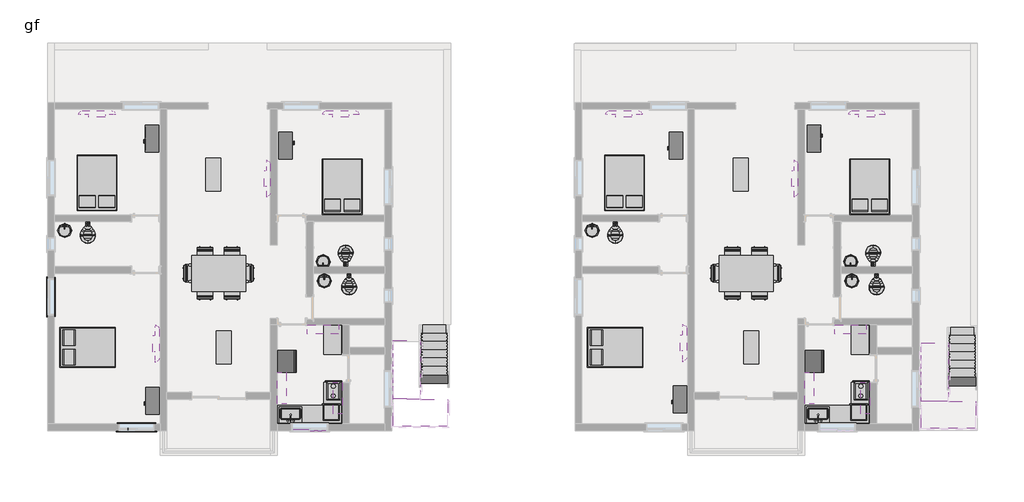
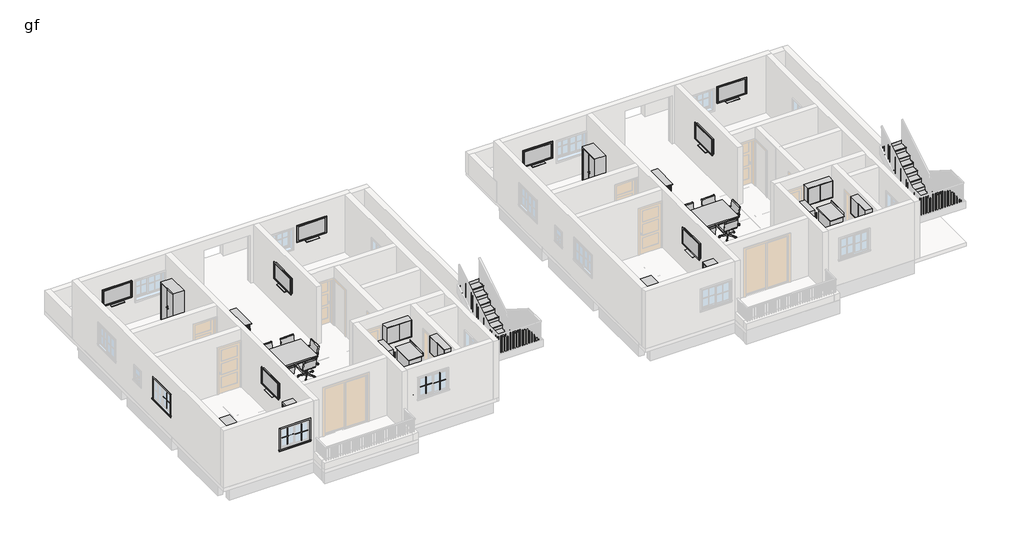
# One storey, part 7 of 8: 56 furniture elements, 23 proxies, 14 flow terminals, 4 stair flights, 2 slabs.
"""IFC4 building model written with IfcOpenShell, lengths in millimetres."""

from ifc_helpers import new_model, si_unit, origin, place, context, project, spatial, transform, mapped, element, save
from components import proxy_3c1fa1d0, proxy_caef4acf, muntin_pattern_2x2_muntin_pattern_2x2_0ac132d2, muntin_pattern_2x2_muntin_pattern_2x2_1fb5fae3, proxy_68898770, proxy_19935bb1, trim_window_exterior_flat_with_sill_c4e67c73, trim_window_exterior_flat_with_sill_729ce974, trim_window_interior_flat_picture_frame_cf1733af, trim_window_interior_flat_picture_frame_5593adf3, flow_terminal_4d548711, flow_terminal_a43f4bde, flow_terminal_3100e559, furniture_6369f5ad, furniture_f415afdb, furniture_97fe820d, furniture_b58f7881, furniture_d3d70ab1, chair_task_chair_task_b7f3823b, chair_task_arms_chair_task_arms_fa5a08ef, furniture_47cc8d9a, furniture_d87d408b, furniture_e7d75d8c, furniture_0b81fedb, furniture_74675f9f, furniture_0bcc43ae, upper_cabinet_sliding_double_door_wall_3e092c2a, non_monolithic_landing_f4ee6888, non_monolithic_landing_6912f083, stair_flight_61f47217, stair_flight_d9814c51, stair_flight_2edfd720, stair_flight_75ff7960

model = new_model("IFC4")

# Units and contexts
model_context = context("Model", 3, world=origin())
ifc_project = project(units=[si_unit("LENGTHUNIT", "METRE", prefix="MILLI")], contexts=[model_context])

# Site, building, storey
site = spatial("IfcSite", under=ifc_project)
building = spatial("IfcBuilding", under=site)
storey = spatial("IfcBuildingStorey", under=building, Name="gf", Elevation=609.6)

# Proxies
placement = place(None, origin())
proxy_shape = proxy_3c1fa1d0(model_context)
element("IfcBuildingElementProxy", 1, Name="Cook Top-2 Unit : 12\" x 18\" 2", ObjectType="Cook Top-2 Unit : 12\" x 18\" 2", at=placement, inside=storey, context=model_context, shape_type="MappedRepresentation", body=[
    mapped(proxy_shape, transform((-6699.3993763, -3292.5061971, 609.6), x_axis=(1.0, 0.0, 0.0), y_axis=(0.0, 1.0, 0.0), z_axis=(0.0, 0.0, 1.0))),
])
element("IfcBuildingElementProxy", 2, Name="Cook Top-2 Unit : 12\" x 18\" 2", ObjectType="Cook Top-2 Unit : 12\" x 18\" 2", at=placement, inside=storey, context=model_context, shape_type="MappedRepresentation", body=[
    mapped(proxy_shape, transform((11175.1761273, -3292.5061971, 609.6), x_axis=(1.0, 0.0, 0.0), y_axis=(0.0, 1.0, 0.0), z_axis=(0.0, 0.0, 1.0))),
])
proxy_2_shape = proxy_caef4acf(model_context)
element("IfcBuildingElementProxy", 3, Name="Cook Top-2 Unit : 16\" x 22\"", ObjectType="Cook Top-2 Unit : 16\" x 22\"", at=placement, inside=storey, context=model_context, shape_type="MappedRepresentation", body=[
    mapped(proxy_2_shape, transform((-6775.5993763, -4038.6311971, 609.6), x_axis=(1.0, 0.0, 0.0), y_axis=(0.0, 1.0, 0.0), z_axis=(0.0, 0.0, 1.0))),
])
element("IfcBuildingElementProxy", 4, Name="Cook Top-2 Unit : 16\" x 22\"", ObjectType="Cook Top-2 Unit : 16\" x 22\"", at=placement, inside=storey, context=model_context, shape_type="MappedRepresentation", body=[
    mapped(proxy_2_shape, transform((-6864.4993763, -4089.4311971, 609.6), x_axis=(1.0, 0.0, 0.0), y_axis=(0.0, 1.0, 0.0), z_axis=(0.0, 0.0, 1.0))),
])
element("IfcBuildingElementProxy", 5, Name="Cook Top-2 Unit : 16\" x 22\"", ObjectType="Cook Top-2 Unit : 16\" x 22\"", at=placement, inside=storey, context=model_context, shape_type="MappedRepresentation", body=[
    mapped(proxy_2_shape, transform((-6699.3993763, -3340.1311971, 609.6), x_axis=(1.0, 0.0, 0.0), y_axis=(0.0, 1.0, 0.0), z_axis=(0.0, 0.0, 1.0))),
])
element("IfcBuildingElementProxy", 6, Name="Cook Top-2 Unit : 16\" x 22\"", ObjectType="Cook Top-2 Unit : 16\" x 22\"", at=placement, inside=storey, context=model_context, shape_type="MappedRepresentation", body=[
    mapped(proxy_2_shape, transform((-6737.4993763, -3556.0311971, 609.6), x_axis=(1.0, 0.0, 0.0), y_axis=(0.0, 1.0, 0.0), z_axis=(0.0, 0.0, 1.0))),
])
element("IfcBuildingElementProxy", 7, Name="Cook Top-2 Unit : 16\" x 22\"", ObjectType="Cook Top-2 Unit : 16\" x 22\"", at=placement, inside=storey, context=model_context, shape_type="MappedRepresentation", body=[
    mapped(proxy_2_shape, transform((11098.9761273, -4038.6311971, 609.6), x_axis=(1.0, 0.0, 0.0), y_axis=(0.0, 1.0, 0.0), z_axis=(0.0, 0.0, 1.0))),
])
element("IfcBuildingElementProxy", 8, Name="Cook Top-2 Unit : 16\" x 22\"", ObjectType="Cook Top-2 Unit : 16\" x 22\"", at=placement, inside=storey, context=model_context, shape_type="MappedRepresentation", body=[
    mapped(proxy_2_shape, transform((11010.0761273, -4089.4311971, 609.6), x_axis=(1.0, 0.0, 0.0), y_axis=(0.0, 1.0, 0.0), z_axis=(0.0, 0.0, 1.0))),
])
element("IfcBuildingElementProxy", 9, Name="Cook Top-2 Unit : 16\" x 22\"", ObjectType="Cook Top-2 Unit : 16\" x 22\"", at=placement, inside=storey, context=model_context, shape_type="MappedRepresentation", body=[
    mapped(proxy_2_shape, transform((11175.1761273, -3340.1311971, 609.6), x_axis=(1.0, 0.0, 0.0), y_axis=(0.0, 1.0, 0.0), z_axis=(0.0, 0.0, 1.0))),
])
element("IfcBuildingElementProxy", 10, Name="Cook Top-2 Unit : 16\" x 22\"", ObjectType="Cook Top-2 Unit : 16\" x 22\"", at=placement, inside=storey, context=model_context, shape_type="MappedRepresentation", body=[
    mapped(proxy_2_shape, transform((11137.0761273, -3556.0311971, 609.6), x_axis=(1.0, 0.0, 0.0), y_axis=(0.0, 1.0, 0.0), z_axis=(0.0, 0.0, 1.0))),
])
muntin_pattern_2x2_muntin_pattern_2x2_shape = muntin_pattern_2x2_muntin_pattern_2x2_0ac132d2(model_context)
element("IfcBuildingElementProxy", 11, Name="Muntin Pattern_2x2 : Muntin Pattern_2x2", ObjectType="Muntin Pattern_2x2 : Muntin Pattern_2x2", at=placement, inside=storey, context=model_context, shape_type="MappedRepresentation", body=[
    mapped(muntin_pattern_2x2_muntin_pattern_2x2_shape, transform((-7707.4618763, -4551.3314015, 1835.15), x_axis=(-1.0, 0.0, 0.0), y_axis=(0.0, -1.0, 0.0), z_axis=(0.0, 0.0, 1.0))),
])
element("IfcBuildingElementProxy", 12, Name="Muntin Pattern_2x2 : Muntin Pattern_2x2", ObjectType="Muntin Pattern_2x2 : Muntin Pattern_2x2", at=placement, inside=storey, context=model_context, shape_type="MappedRepresentation", body=[
    mapped(muntin_pattern_2x2_muntin_pattern_2x2_shape, transform((-7139.1368763, -4595.7814015, 1835.15), x_axis=(-1.0, 0.0, 0.0), y_axis=(0.0, -1.0, 0.0), z_axis=(0.0, 0.0, 1.0))),
])
element("IfcBuildingElementProxy", 13, Name="Muntin Pattern_2x2 : Muntin Pattern_2x2", ObjectType="Muntin Pattern_2x2 : Muntin Pattern_2x2", at=placement, inside=storey, context=model_context, shape_type="MappedRepresentation", body=[
    mapped(muntin_pattern_2x2_muntin_pattern_2x2_shape, transform((-13574.8618763, -4551.3314015, 1606.55), x_axis=(-1.0, 0.0, 0.0), y_axis=(0.0, -1.0, 0.0), z_axis=(0.0, 0.0, 1.0))),
])
element("IfcBuildingElementProxy", 14, Name="Muntin Pattern_2x2 : Muntin Pattern_2x2", ObjectType="Muntin Pattern_2x2 : Muntin Pattern_2x2", at=placement, inside=storey, context=model_context, shape_type="MappedRepresentation", body=[
    mapped(muntin_pattern_2x2_muntin_pattern_2x2_shape, transform((-13006.5368763, -4595.7814015, 1606.55), x_axis=(-1.0, 0.0, 0.0), y_axis=(0.0, -1.0, 0.0), z_axis=(0.0, 0.0, 1.0))),
])
muntin_pattern_2x2_muntin_pattern_2x2_2_shape = muntin_pattern_2x2_muntin_pattern_2x2_1fb5fae3(model_context)
element("IfcBuildingElementProxy", 15, Name="Muntin Pattern_2x2 : Muntin Pattern_2x2", ObjectType="Muntin Pattern_2x2 : Muntin Pattern_2x2", at=placement, inside=storey, context=model_context, shape_type="MappedRepresentation", body=[
    mapped(muntin_pattern_2x2_muntin_pattern_2x2_2_shape, transform((-16246.6243763, -355.5689015, 1606.55), x_axis=(0.0, -1.0, 0.0), y_axis=(1.0, 0.0, 0.0), z_axis=(0.0, 0.0, 1.0))),
])
proxy_3_shape = proxy_68898770(model_context)
element("IfcBuildingElementProxy", 16, Name="Oven Single-Built-in : 21\" x 23 1/2\" x 21\"", ObjectType="Oven Single-Built-in : 21\" x 23 1/2\" x 21\"", at=placement, inside=storey, context=model_context, shape_type="MappedRepresentation", body=[
    mapped(proxy_3_shape, transform((-6728.2243036, -3854.6405426, 1422.4), x_axis=(-1.0, 0.0, 0.0), y_axis=(0.0, -1.0, 0.0), z_axis=(0.0, 0.0, 1.0))),
])
element("IfcBuildingElementProxy", 17, Name="Oven Single-Built-in : 21\" x 23 1/2\" x 21\"", ObjectType="Oven Single-Built-in : 21\" x 23 1/2\" x 21\"", at=placement, inside=storey, context=model_context, shape_type="MappedRepresentation", body=[
    mapped(proxy_3_shape, transform((11146.3512, -3854.6405426, 1422.4), x_axis=(-1.0, 0.0, 0.0), y_axis=(0.0, -1.0, 0.0), z_axis=(0.0, 0.0, 1.0))),
])
proxy_4_shape = proxy_19935bb1(model_context)
element("IfcBuildingElementProxy", 18, Name="Refrigerator-Built-in : 30\" x 24\" LH", ObjectType="Refrigerator-Built-in : 30\" x 24\" LH", at=placement, inside=storey, context=model_context, shape_type="MappedRepresentation", body=[
    mapped(proxy_4_shape, transform((-8238.0754048, -2262.1564015, 609.6), x_axis=(0.0, 1.0, 0.0), y_axis=(-1.0, 0.0, 0.0), z_axis=(0.0, 0.0, 1.0))),
])
element("IfcBuildingElementProxy", 19, Name="Refrigerator-Built-in : 30\" x 24\" LH", ObjectType="Refrigerator-Built-in : 30\" x 24\" LH", at=placement, inside=storey, context=model_context, shape_type="MappedRepresentation", body=[
    mapped(proxy_4_shape, transform((9636.5000988, -2262.1564015, 609.6), x_axis=(0.0, 1.0, 0.0), y_axis=(-1.0, 0.0, 0.0), z_axis=(0.0, 0.0, 1.0))),
])
trim_window_exterior_flat_with_sill_shape = trim_window_exterior_flat_with_sill_c4e67c73(model_context)
element("IfcBuildingElementProxy", 20, Name="Trim-Window-Exterior-Flat : with Sill", ObjectType="Trim-Window-Exterior-Flat : with Sill", at=placement, inside=storey, context=model_context, shape_type="MappedRepresentation", body=[
    mapped(trim_window_exterior_flat_with_sill_shape, transform((-13290.6993763, -4605.3064015, 2438.4), x_axis=(1.0, 0.0, 0.0), y_axis=(0.0, 0.0, 1.0), z_axis=(0.0, -1.0, 0.0))),
])
trim_window_exterior_flat_with_sill_2_shape = trim_window_exterior_flat_with_sill_729ce974(model_context)
element("IfcBuildingElementProxy", 21, Name="Trim-Window-Exterior-Flat : with Sill", ObjectType="Trim-Window-Exterior-Flat : with Sill", at=placement, inside=storey, context=model_context, shape_type="MappedRepresentation", body=[
    mapped(trim_window_exterior_flat_with_sill_2_shape, transform((-16300.5993763, -71.4064015, 2438.4), x_axis=(0.0, 1.0, 0.0), y_axis=(0.0, 0.0, -1.0), z_axis=(-1.0, 0.0, 0.0))),
])
trim_window_interior_flat_picture_frame_shape = trim_window_interior_flat_picture_frame_cf1733af(model_context)
element("IfcBuildingElementProxy", 22, Name="Trim-Window-Interior-Flat : Picture Frame", ObjectType="Trim-Window-Interior-Flat : Picture Frame", at=placement, inside=storey, context=model_context, shape_type="MappedRepresentation", body=[
    mapped(trim_window_interior_flat_picture_frame_shape, transform((-13290.6993763, -4376.7064015, 2438.4), x_axis=(-1.0, 0.0, 0.0), y_axis=(0.0, 0.0, 1.0), z_axis=(0.0, 1.0, 0.0))),
])
trim_window_interior_flat_picture_frame_2_shape = trim_window_interior_flat_picture_frame_5593adf3(model_context)
element("IfcBuildingElementProxy", 23, Name="Trim-Window-Interior-Flat : Picture Frame", ObjectType="Trim-Window-Interior-Flat : Picture Frame", at=placement, inside=storey, context=model_context, shape_type="MappedRepresentation", body=[
    mapped(trim_window_interior_flat_picture_frame_2_shape, transform((-16071.9993763, -71.4064015, 2438.4), x_axis=(0.0, -1.0, 0.0), y_axis=(0.0, 0.0, -1.0), z_axis=(1.0, 0.0, 0.0))),
])

# Flow terminals
flow_terminal_shape = flow_terminal_4d548711(model_context)
element("IfcFlowTerminal", 24, ObjectType="Sink Kitchen-Single : 30\" x 21\"", at=placement, inside=storey, context=model_context, shape_type="MappedRepresentation", body=[
    mapped(flow_terminal_shape, transform((-8055.3101357, -4069.5610004, 609.6), x_axis=(-1.0, 0.0, 0.0), y_axis=(0.0, -1.0, 0.0), z_axis=(0.0, 0.0, 1.0))),
])
element("IfcFlowTerminal", 25, ObjectType="Sink Kitchen-Single : 30\" x 21\"", at=placement, inside=storey, context=model_context, shape_type="MappedRepresentation", body=[
    mapped(flow_terminal_shape, transform((9819.2653679, -4069.5610004, 609.6), x_axis=(-1.0, 0.0, 0.0), y_axis=(0.0, -1.0, 0.0), z_axis=(0.0, 0.0, 1.0))),
])
flow_terminal_2_shape = flow_terminal_a43f4bde(model_context)
element("IfcFlowTerminal", 26, ObjectType="Sink Vanity-Round : 19\" x 19\"", at=placement, inside=storey, context=model_context, shape_type="MappedRepresentation", body=[
    mapped(flow_terminal_2_shape, transform((-15825.7511169, 2099.027665, 609.6), x_axis=(1.0, 0.0, 0.0), y_axis=(0.0, 1.0, 0.0), z_axis=(0.0, 0.0, 1.0))),
])
element("IfcFlowTerminal", 27, ObjectType="Sink Vanity-Round : 19\" x 19\"", at=placement, inside=storey, context=model_context, shape_type="MappedRepresentation", body=[
    mapped(flow_terminal_2_shape, transform((-6868.8660625, 1205.7175518, 609.6), x_axis=(-0.9999644866359478, 0.008427660820502282, 0.0), y_axis=(-0.008427660820502282, -0.9999644866359478, 0.0), z_axis=(0.0, 0.0, 1.0))),
])
element("IfcFlowTerminal", 28, ObjectType="Sink Vanity-Round : 19\" x 19\"", at=placement, inside=storey, context=model_context, shape_type="MappedRepresentation", body=[
    mapped(flow_terminal_2_shape, transform((-7024.6511169, 390.0887767, 609.6), x_axis=(1.0, 0.0, 0.0), y_axis=(0.0, 1.0, 0.0), z_axis=(0.0, 0.0, 1.0))),
])
element("IfcFlowTerminal", 29, ObjectType="Sink Vanity-Round : 19\" x 19\"", at=placement, inside=storey, context=model_context, shape_type="MappedRepresentation", body=[
    mapped(flow_terminal_2_shape, transform((2048.8243868, 2099.027665, 609.6), x_axis=(1.0, 0.0, 0.0), y_axis=(0.0, 1.0, 0.0), z_axis=(0.0, 0.0, 1.0))),
])
element("IfcFlowTerminal", 30, ObjectType="Sink Vanity-Round : 19\" x 19\"", at=placement, inside=storey, context=model_context, shape_type="MappedRepresentation", body=[
    mapped(flow_terminal_2_shape, transform((11005.7094411, 1205.7175518, 609.6), x_axis=(-0.999964486635994, 0.008427660815032186, 0.0), y_axis=(-0.008427660815032186, -0.999964486635994, 0.0), z_axis=(0.0, 0.0, 1.0))),
])
element("IfcFlowTerminal", 31, ObjectType="Sink Vanity-Round : 19\" x 19\"", at=placement, inside=storey, context=model_context, shape_type="MappedRepresentation", body=[
    mapped(flow_terminal_2_shape, transform((10849.9243868, 390.0887767, 609.6), x_axis=(1.0, 0.0, 0.0), y_axis=(0.0, 1.0, 0.0), z_axis=(0.0, 0.0, 1.0))),
])
flow_terminal_3_shape = flow_terminal_3100e559(model_context)
element("IfcFlowTerminal", 32, ObjectType="Toilet-Commercial-Wall-3D : 15\" Seat Height", at=placement, inside=storey, context=model_context, shape_type="MappedRepresentation", body=[
    mapped(flow_terminal_3_shape, transform((-5684.8962225, 842.9935985, 609.6), x_axis=(-1.0, 0.0, 0.0), y_axis=(0.0, -1.0, 0.0), z_axis=(0.0, 0.0, 1.0))),
])
element("IfcFlowTerminal", 33, ObjectType="Toilet-Commercial-Wall-3D : 15\" Seat Height", at=placement, inside=storey, context=model_context, shape_type="MappedRepresentation", body=[
    mapped(flow_terminal_3_shape, transform((-6609.0025301, 842.9935985, 609.6), x_axis=(1.0, 0.0, 0.0), y_axis=(0.0, 1.0, 0.0), z_axis=(0.0, 0.0, 1.0))),
])
element("IfcFlowTerminal", 34, ObjectType="Toilet-Commercial-Wall-3D : 15\" Seat Height", at=placement, inside=storey, context=model_context, shape_type="MappedRepresentation", body=[
    mapped(flow_terminal_3_shape, transform((-14536.7962225, 2595.5935985, 609.6), x_axis=(-1.0, 0.0, 0.0), y_axis=(0.0, -1.0, 0.0), z_axis=(0.0, 0.0, 1.0))),
])
element("IfcFlowTerminal", 35, ObjectType="Toilet-Commercial-Wall-3D : 15\" Seat Height", at=placement, inside=storey, context=model_context, shape_type="MappedRepresentation", body=[
    mapped(flow_terminal_3_shape, transform((12189.6792812, 842.9935985, 609.6), x_axis=(-1.0, 0.0, 0.0), y_axis=(0.0, -1.0, 0.0), z_axis=(0.0, 0.0, 1.0))),
])
element("IfcFlowTerminal", 36, ObjectType="Toilet-Commercial-Wall-3D : 15\" Seat Height", at=placement, inside=storey, context=model_context, shape_type="MappedRepresentation", body=[
    mapped(flow_terminal_3_shape, transform((11265.5729735, 842.9935985, 609.6), x_axis=(1.0, 0.0, 0.0), y_axis=(0.0, 1.0, 0.0), z_axis=(0.0, 0.0, 1.0))),
])
element("IfcFlowTerminal", 37, ObjectType="Toilet-Commercial-Wall-3D : 15\" Seat Height", at=placement, inside=storey, context=model_context, shape_type="MappedRepresentation", body=[
    mapped(flow_terminal_3_shape, transform((3337.7792812, 2595.5935985, 609.6), x_axis=(-1.0, 0.0, 0.0), y_axis=(0.0, -1.0, 0.0), z_axis=(0.0, 0.0, 1.0))),
])

# Furniture
furniture_shape = furniture_6369f5ad(model_context)
element("IfcFurniture", 38, ObjectType="Base Cabinet-Acid Storage Unit : 30\" 2", at=placement, inside=storey, context=model_context, shape_type="MappedRepresentation", body=[
    mapped(furniture_shape, transform((-6343.7993763, -3202.2686966, 609.6), x_axis=(0.0, -1.0, 0.0), y_axis=(1.0, 0.0, 0.0), z_axis=(0.0, 0.0, 1.0))),
])
element("IfcFurniture", 39, ObjectType="Base Cabinet-Acid Storage Unit : 30\" 2", at=placement, inside=storey, context=model_context, shape_type="MappedRepresentation", body=[
    mapped(furniture_shape, transform((11530.7761273, -3202.2686966, 609.6), x_axis=(0.0, -1.0, 0.0), y_axis=(1.0, 0.0, 0.0), z_axis=(0.0, 0.0, 1.0))),
])
furniture_2_shape = furniture_f415afdb(model_context)
element("IfcFurniture", 40, ObjectType="Base Cabinet-Combo01 : 30\" 2", at=placement, inside=storey, context=model_context, shape_type="MappedRepresentation", body=[
    mapped(furniture_2_shape, transform((-6318.3993763, -1386.1686966, 609.6), x_axis=(0.0, -1.0, 0.0), y_axis=(1.0, 0.0, 0.0), z_axis=(0.0, 0.0, 1.0))),
])
element("IfcFurniture", 41, ObjectType="Base Cabinet-Combo01 : 30\" 2", at=placement, inside=storey, context=model_context, shape_type="MappedRepresentation", body=[
    mapped(furniture_2_shape, transform((11556.1761273, -1386.1686966, 609.6), x_axis=(0.0, -1.0, 0.0), y_axis=(1.0, 0.0, 0.0), z_axis=(0.0, 0.0, 1.0))),
])
furniture_3_shape = furniture_97fe820d(model_context)
element("IfcFurniture", 42, ObjectType="Base Cabinet-Corner Unit-Square : 36\"", at=placement, inside=storey, context=model_context, shape_type="MappedRepresentation", body=[
    mapped(furniture_3_shape, transform((-6318.3993763, -3849.9686966, 609.6), x_axis=(0.0, -1.0, 0.0), y_axis=(1.0, 0.0, 0.0), z_axis=(0.0, 0.0, 1.0))),
])
element("IfcFurniture", 43, ObjectType="Base Cabinet-Corner Unit-Square : 36\"", at=placement, inside=storey, context=model_context, shape_type="MappedRepresentation", body=[
    mapped(furniture_3_shape, transform((11556.1761273, -3849.9686966, 609.6), x_axis=(0.0, -1.0, 0.0), y_axis=(1.0, 0.0, 0.0), z_axis=(0.0, 0.0, 1.0))),
])
furniture_4_shape = furniture_b58f7881(model_context)
element("IfcFurniture", 44, ObjectType="Bed-Box : Double 53\" x 74\"", at=placement, inside=storey, context=model_context, shape_type="MappedRepresentation", body=[
    mapped(furniture_4_shape, transform((-14292.2379089, 3557.6185064, 609.6), x_axis=(-1.0, 0.0, 0.0), y_axis=(0.0, -1.0, 0.0), z_axis=(0.0, 0.0, 1.0))),
])
element("IfcFurniture", 45, ObjectType="Bed-Box : Double 53\" x 74\"", at=placement, inside=storey, context=model_context, shape_type="MappedRepresentation", body=[
    mapped(furniture_4_shape, transform((-15182.9191795, -2125.0588605, 609.6), x_axis=(0.0, 1.0, 0.0), y_axis=(-1.0, 0.0, 0.0), z_axis=(0.0, 0.0, 1.0))),
])
element("IfcFurniture", 46, ObjectType="Bed-Box : Double 53\" x 74\"", at=placement, inside=storey, context=model_context, shape_type="MappedRepresentation", body=[
    mapped(furniture_4_shape, transform((-5979.2469173, 3433.3274594, 609.6), x_axis=(-1.0, 0.0, 0.0), y_axis=(0.0, -1.0, 0.0), z_axis=(0.0, 0.0, 1.0))),
])
element("IfcFurniture", 47, ObjectType="Bed-Box : Double 53\" x 74\"", at=placement, inside=storey, context=model_context, shape_type="MappedRepresentation", body=[
    mapped(furniture_4_shape, transform((3582.3375948, 3557.6185064, 609.6), x_axis=(-1.0, 0.0, 0.0), y_axis=(0.0, -1.0, 0.0), z_axis=(0.0, 0.0, 1.0))),
])
element("IfcFurniture", 48, ObjectType="Bed-Box : Double 53\" x 74\"", at=placement, inside=storey, context=model_context, shape_type="MappedRepresentation", body=[
    mapped(furniture_4_shape, transform((2691.6563242, -2125.0588605, 609.6), x_axis=(0.0, 1.0, 0.0), y_axis=(-1.0, 0.0, 0.0), z_axis=(0.0, 0.0, 1.0))),
])
element("IfcFurniture", 49, ObjectType="Bed-Box : Double 53\" x 74\"", at=placement, inside=storey, context=model_context, shape_type="MappedRepresentation", body=[
    mapped(furniture_4_shape, transform((11895.3285864, 3433.3274594, 609.6), x_axis=(-1.0, 0.0, 0.0), y_axis=(0.0, -1.0, 0.0), z_axis=(0.0, 0.0, 1.0))),
])
furniture_5_shape = furniture_d3d70ab1(model_context)
element("IfcFurniture", 50, ObjectType="Cabinet-Storage : 36\" x 18\" x 72\"", at=placement, inside=storey, context=model_context, shape_type="MappedRepresentation", body=[
    mapped(furniture_5_shape, transform((-12757.2993763, 5305.7833167, 609.6), x_axis=(0.0, -1.0, 0.0), y_axis=(1.0, 0.0, 0.0), z_axis=(0.0, 0.0, 1.0))),
])
element("IfcFurniture", 51, ObjectType="Cabinet-Storage : 36\" x 18\" x 72\"", at=placement, inside=storey, context=model_context, shape_type="MappedRepresentation", body=[
    mapped(furniture_5_shape, transform((-8236.2515468, 5059.3935985, 609.6), x_axis=(0.0, 1.0, 0.0), y_axis=(-1.0, 0.0, 0.0), z_axis=(0.0, 0.0, 1.0))),
])
element("IfcFurniture", 52, ObjectType="Cabinet-Storage : 36\" x 18\" x 72\"", at=placement, inside=storey, context=model_context, shape_type="MappedRepresentation", body=[
    mapped(furniture_5_shape, transform((-12748.5420807, -3590.3671413, 609.6), x_axis=(0.0, -1.0, 0.0), y_axis=(1.0, 0.0, 0.0), z_axis=(0.0, 0.0, 1.0))),
])
element("IfcFurniture", 53, ObjectType="Cabinet-Storage : 36\" x 18\" x 72\"", at=placement, inside=storey, context=model_context, shape_type="MappedRepresentation", body=[
    mapped(furniture_5_shape, transform((4992.1783017, 5059.3935985, 609.6), x_axis=(0.0, -1.0, 0.0), y_axis=(1.0, 0.0, 0.0), z_axis=(0.0, 0.0, 1.0))),
])
element("IfcFurniture", 54, ObjectType="Cabinet-Storage : 36\" x 18\" x 72\"", at=placement, inside=storey, context=model_context, shape_type="MappedRepresentation", body=[
    mapped(furniture_5_shape, transform((5126.8930163, -3538.5064015, 609.6), x_axis=(0.0, -1.0, 0.0), y_axis=(1.0, 0.0, 0.0), z_axis=(0.0, 0.0, 1.0))),
])
element("IfcFurniture", 55, ObjectType="Cabinet-Storage : 36\" x 18\" x 72\"", at=placement, inside=storey, context=model_context, shape_type="MappedRepresentation", body=[
    mapped(furniture_5_shape, transform((9660.8090799, 5305.7833167, 609.6), x_axis=(0.0, 1.0, 0.0), y_axis=(-1.0, 0.0, 0.0), z_axis=(0.0, 0.0, 1.0))),
])
chair_task_chair_task_shape = chair_task_chair_task_b7f3823b(model_context)
element("IfcFurniture", 56, ObjectType="Chair-Task : Chair-Task", at=placement, inside=storey, context=model_context, shape_type="MappedRepresentation", body=[
    mapped(chair_task_chair_task_shape, transform((-9911.2085566, 1357.2395001, 609.6), x_axis=(-1.0, 0.0, 0.0), y_axis=(0.0, -1.0, 0.0), z_axis=(0.0, 0.0, 1.0))),
])
element("IfcFurniture", 57, ObjectType="Chair-Task : Chair-Task", at=placement, inside=storey, context=model_context, shape_type="MappedRepresentation", body=[
    mapped(chair_task_chair_task_shape, transform((-10193.190196, 100.1476968, 609.6), x_axis=(1.0, 0.0, 0.0), y_axis=(0.0, 1.0, 0.0), z_axis=(0.0, 0.0, 1.0))),
])
element("IfcFurniture", 58, ObjectType="Chair-Task : Chair-Task", at=placement, inside=storey, context=model_context, shape_type="MappedRepresentation", body=[
    mapped(chair_task_chair_task_shape, transform((-10825.6085566, 1357.2395001, 609.6), x_axis=(-1.0, 0.0, 0.0), y_axis=(0.0, -1.0, 0.0), z_axis=(0.0, 0.0, 1.0))),
])
element("IfcFurniture", 59, ObjectType="Chair-Task : Chair-Task", at=placement, inside=storey, context=model_context, shape_type="MappedRepresentation", body=[
    mapped(chair_task_chair_task_shape, transform((-11107.590196, 100.1476968, 609.6), x_axis=(1.0, 0.0, 0.0), y_axis=(0.0, 1.0, 0.0), z_axis=(0.0, 0.0, 1.0))),
])
element("IfcFurniture", 60, ObjectType="Chair-Task : Chair-Task", at=placement, inside=storey, context=model_context, shape_type="MappedRepresentation", body=[
    mapped(chair_task_chair_task_shape, transform((7963.366947, 1357.2395001, 609.6), x_axis=(-1.0, 0.0, 0.0), y_axis=(0.0, -1.0, 0.0), z_axis=(0.0, 0.0, 1.0))),
])
element("IfcFurniture", 61, ObjectType="Chair-Task : Chair-Task", at=placement, inside=storey, context=model_context, shape_type="MappedRepresentation", body=[
    mapped(chair_task_chair_task_shape, transform((7681.3853077, 100.1476968, 609.6), x_axis=(1.0, 0.0, 0.0), y_axis=(0.0, 1.0, 0.0), z_axis=(0.0, 0.0, 1.0))),
])
element("IfcFurniture", 62, ObjectType="Chair-Task : Chair-Task", at=placement, inside=storey, context=model_context, shape_type="MappedRepresentation", body=[
    mapped(chair_task_chair_task_shape, transform((7048.966947, 1357.2395001, 609.6), x_axis=(-1.0, 0.0, 0.0), y_axis=(0.0, -1.0, 0.0), z_axis=(0.0, 0.0, 1.0))),
])
element("IfcFurniture", 63, ObjectType="Chair-Task : Chair-Task", at=placement, inside=storey, context=model_context, shape_type="MappedRepresentation", body=[
    mapped(chair_task_chair_task_shape, transform((6766.9853077, 100.1476968, 609.6), x_axis=(1.0, 0.0, 0.0), y_axis=(0.0, 1.0, 0.0), z_axis=(0.0, 0.0, 1.0))),
])
chair_task_arms_chair_task_arms_shape = chair_task_arms_chair_task_arms_fa5a08ef(model_context)
element("IfcFurniture", 64, ObjectType="Chair-Task Arms : Chair-Task Arms", at=placement, inside=storey, context=model_context, shape_type="MappedRepresentation", body=[
    mapped(chair_task_arms_chair_task_arms_shape, transform((-11442.7452779, 869.6844182, 609.6), x_axis=(0.0, -1.0, 0.0), y_axis=(1.0, 0.0, 0.0), z_axis=(0.0, 0.0, 1.0))),
])
element("IfcFurniture", 65, ObjectType="Chair-Task Arms : Chair-Task Arms", at=placement, inside=storey, context=model_context, shape_type="MappedRepresentation", body=[
    mapped(chair_task_arms_chair_task_arms_shape, transform((-9576.0534746, 587.7027788, 609.6), x_axis=(0.0, 1.0, 0.0), y_axis=(-1.0, 0.0, 0.0), z_axis=(0.0, 0.0, 1.0))),
])
element("IfcFurniture", 66, ObjectType="Chair-Task Arms : Chair-Task Arms", at=placement, inside=storey, context=model_context, shape_type="MappedRepresentation", body=[
    mapped(chair_task_arms_chair_task_arms_shape, transform((6431.8302257, 869.6844182, 609.6), x_axis=(0.0, -1.0, 0.0), y_axis=(1.0, 0.0, 0.0), z_axis=(0.0, 0.0, 1.0))),
])
element("IfcFurniture", 67, ObjectType="Chair-Task Arms : Chair-Task Arms", at=placement, inside=storey, context=model_context, shape_type="MappedRepresentation", body=[
    mapped(chair_task_arms_chair_task_arms_shape, transform((8298.522029, 587.7027788, 609.6), x_axis=(0.0, 1.0, 0.0), y_axis=(-1.0, 0.0, 0.0), z_axis=(0.0, 0.0, 1.0))),
])
furniture_6_shape = furniture_47cc8d9a(model_context)
element("IfcFurniture", 68, ObjectType="Counter Top : 24\" Depth", at=placement, inside=storey, context=model_context, shape_type="MappedRepresentation", body=[
    mapped(furniture_6_shape, transform((-6318.3993763, -2224.3686966, 609.6), x_axis=(0.0, -1.0, 0.0), y_axis=(1.0, 0.0, 0.0), z_axis=(0.0, 0.0, 1.0))),
])
element("IfcFurniture", 69, ObjectType="Counter Top : 24\" Depth", at=placement, inside=storey, context=model_context, shape_type="MappedRepresentation", body=[
    mapped(furniture_6_shape, transform((11556.1761273, -2224.3686966, 609.6), x_axis=(0.0, -1.0, 0.0), y_axis=(1.0, 0.0, 0.0), z_axis=(0.0, 0.0, 1.0))),
])
furniture_7_shape = furniture_d87d408b(model_context)
element("IfcFurniture", 70, ObjectType="Counter Top : 24\" Depth", at=placement, inside=storey, context=model_context, shape_type="MappedRepresentation", body=[
    mapped(furniture_7_shape, transform((-6318.3993763, -4167.4686966, 609.6), x_axis=(0.0, -1.0, 0.0), y_axis=(1.0, 0.0, 0.0), z_axis=(0.0, 0.0, 1.0))),
])
element("IfcFurniture", 71, ObjectType="Counter Top : 24\" Depth", at=placement, inside=storey, context=model_context, shape_type="MappedRepresentation", body=[
    mapped(furniture_7_shape, transform((11556.1761273, -4167.4686966, 609.6), x_axis=(0.0, -1.0, 0.0), y_axis=(1.0, 0.0, 0.0), z_axis=(0.0, 0.0, 1.0))),
])
furniture_8_shape = furniture_e7d75d8c(model_context)
element("IfcFurniture", 72, ObjectType="Counter Top w Sink Hole : 24\" Depth", at=placement, inside=storey, context=model_context, shape_type="MappedRepresentation", body=[
    mapped(furniture_8_shape, transform((-7518.8616714, -4376.7064015, 609.6), x_axis=(-1.0, 0.0, 0.0), y_axis=(0.0, -1.0, 0.0), z_axis=(0.0, 0.0, 1.0))),
])
element("IfcFurniture", 73, ObjectType="Counter Top w Sink Hole : 24\" Depth", at=placement, inside=storey, context=model_context, shape_type="MappedRepresentation", body=[
    mapped(furniture_8_shape, transform((10355.7138323, -4376.7064015, 609.6), x_axis=(-1.0, 0.0, 0.0), y_axis=(0.0, -1.0, 0.0), z_axis=(0.0, 0.0, 1.0))),
])
furniture_9_shape = furniture_0b81fedb(model_context)
element("IfcFurniture", 74, ObjectType="TV - Flat Screen : 50\"", at=placement, inside=storey, context=model_context, shape_type="MappedRepresentation", body=[
    mapped(furniture_9_shape, transform((-8815.3379999, 3937.8490843, 1828.8), x_axis=(0.0, -1.0, 0.0), y_axis=(1.0, 0.0, 0.0), z_axis=(0.0, 0.0, 1.0))),
])
element("IfcFurniture", 75, ObjectType="TV - Flat Screen : 50\"", at=placement, inside=storey, context=model_context, shape_type="MappedRepresentation", body=[
    mapped(furniture_9_shape, transform((9059.2375037, 3937.8490843, 1828.8), x_axis=(0.0, -1.0, 0.0), y_axis=(1.0, 0.0, 0.0), z_axis=(0.0, 0.0, 1.0))),
])
element("IfcFurniture", 76, ObjectType="TV - Flat Screen : 50\"", at=placement, inside=storey, context=model_context, shape_type="MappedRepresentation", body=[
    mapped(furniture_9_shape, transform((-14627.4458537, 6186.2439145, 1828.8), x_axis=(1.0, 0.0, 0.0), y_axis=(0.0, 1.0, 0.0), z_axis=(0.0, 0.0, 1.0))),
])
element("IfcFurniture", 77, ObjectType="TV - Flat Screen : 50\"", at=placement, inside=storey, context=model_context, shape_type="MappedRepresentation", body=[
    mapped(furniture_9_shape, transform((-12581.2234035, -1662.8509157, 1828.8), x_axis=(0.0, -1.0, 0.0), y_axis=(1.0, 0.0, 0.0), z_axis=(0.0, 0.0, 1.0))),
])
element("IfcFurniture", 78, ObjectType="TV - Flat Screen : 50\"", at=placement, inside=storey, context=model_context, shape_type="MappedRepresentation", body=[
    mapped(furniture_9_shape, transform((-6365.2548621, 6186.2439145, 1828.8), x_axis=(1.0, 0.0, 0.0), y_axis=(0.0, 1.0, 0.0), z_axis=(0.0, 0.0, 1.0))),
])
element("IfcFurniture", 79, ObjectType="TV - Flat Screen : 50\"", at=placement, inside=storey, context=model_context, shape_type="MappedRepresentation", body=[
    mapped(furniture_9_shape, transform((3226.0357212, 6186.2439145, 1828.8), x_axis=(1.0, 0.0, 0.0), y_axis=(0.0, 1.0, 0.0), z_axis=(0.0, 0.0, 1.0))),
])
element("IfcFurniture", 80, ObjectType="TV - Flat Screen : 50\"", at=placement, inside=storey, context=model_context, shape_type="MappedRepresentation", body=[
    mapped(furniture_9_shape, transform((11458.5206415, 6186.2439145, 1828.8), x_axis=(1.0, 0.0, 0.0), y_axis=(0.0, 1.0, 0.0), z_axis=(0.0, 0.0, 1.0))),
])
element("IfcFurniture", 81, ObjectType="TV - Flat Screen : 50\"", at=placement, inside=storey, context=model_context, shape_type="MappedRepresentation", body=[
    mapped(furniture_9_shape, transform((5293.3521002, -1637.4509157, 1828.8), x_axis=(0.0, -1.0, 0.0), y_axis=(1.0, 0.0, 0.0), z_axis=(0.0, 0.0, 1.0))),
])
furniture_10_shape = furniture_74675f9f(model_context)
element("IfcFurniture", 82, ObjectType="Table-Coffee Mission : 44\" x 20\"", at=placement, inside=storey, context=model_context, shape_type="MappedRepresentation", body=[
    mapped(furniture_10_shape, transform((-10683.4908966, 4085.6049296, 609.6), x_axis=(0.0, 1.0, 0.0), y_axis=(-1.0, 0.0, 0.0), z_axis=(0.0, 0.0, 1.0))),
])
element("IfcFurniture", 83, ObjectType="Table-Coffee Mission : 44\" x 20\"", at=placement, inside=storey, context=model_context, shape_type="MappedRepresentation", body=[
    mapped(furniture_10_shape, transform((-10337.6073421, -1785.9064015, 609.6), x_axis=(0.0, 1.0, 0.0), y_axis=(-1.0, 0.0, 0.0), z_axis=(0.0, 0.0, 1.0))),
])
element("IfcFurniture", 84, ObjectType="Table-Coffee Mission : 44\" x 20\"", at=placement, inside=storey, context=model_context, shape_type="MappedRepresentation", body=[
    mapped(furniture_10_shape, transform((7191.084607, 4085.6049296, 609.6), x_axis=(0.0, 1.0, 0.0), y_axis=(-1.0, 0.0, 0.0), z_axis=(0.0, 0.0, 1.0))),
])
element("IfcFurniture", 85, ObjectType="Table-Coffee Mission : 44\" x 20\"", at=placement, inside=storey, context=model_context, shape_type="MappedRepresentation", body=[
    mapped(furniture_10_shape, transform((7536.9681616, -1785.9064015, 609.6), x_axis=(0.0, 1.0, 0.0), y_axis=(-1.0, 0.0, 0.0), z_axis=(0.0, 0.0, 1.0))),
])
furniture_11_shape = furniture_0bcc43ae(model_context)
element("IfcFurniture", 86, ObjectType="Table-Conference2 w Chairs : 48\" x 144\"", at=placement, inside=storey, context=model_context, shape_type="MappedRepresentation", body=[
    mapped(furniture_11_shape, transform((-10509.3993763, 728.6935985, 609.6), x_axis=(1.0, 0.0, 0.0), y_axis=(0.0, 1.0, 0.0), z_axis=(0.0, 0.0, 1.0))),
])
element("IfcFurniture", 87, ObjectType="Table-Conference2 w Chairs : 48\" x 144\"", at=placement, inside=storey, context=model_context, shape_type="MappedRepresentation", body=[
    mapped(furniture_11_shape, transform((7365.1761273, 728.6935985, 609.6), x_axis=(1.0, 0.0, 0.0), y_axis=(0.0, 1.0, 0.0), z_axis=(0.0, 0.0, 1.0))),
])
upper_cabinet_sliding_double_door_wall_shape = upper_cabinet_sliding_double_door_wall_3e092c2a(model_context)
element("IfcFurniture", 88, ObjectType="Upper Cabinet-Sliding Double Door-Wall", at=placement, inside=storey, context=model_context, shape_type="MappedRepresentation", body=[
    mapped(upper_cabinet_sliding_double_door_wall_shape, transform((-6204.0993763, -3530.1775643, 952.5), x_axis=(0.0, 1.0, 0.0), y_axis=(-1.0, 0.0, 0.0), z_axis=(0.0, 0.0, 1.0))),
])
element("IfcFurniture", 89, ObjectType="Upper Cabinet-Sliding Double Door-Wall", at=placement, inside=storey, context=model_context, shape_type="MappedRepresentation", body=[
    mapped(upper_cabinet_sliding_double_door_wall_shape, transform((-6936.3282135, -909.6064015, 609.6), x_axis=(-1.0, 0.0, 0.0), y_axis=(0.0, -1.0, 0.0), z_axis=(0.0, 0.0, 1.0))),
])
element("IfcFurniture", 90, ObjectType="Upper Cabinet-Sliding Double Door-Wall", at=placement, inside=storey, context=model_context, shape_type="MappedRepresentation", body=[
    mapped(upper_cabinet_sliding_double_door_wall_shape, transform((-8642.4993763, -3140.4352387, 609.6), x_axis=(0.0, -1.0, 0.0), y_axis=(1.0, 0.0, 0.0), z_axis=(0.0, 0.0, 1.0))),
])
element("IfcFurniture", 91, ObjectType="Upper Cabinet-Sliding Double Door-Wall", at=placement, inside=storey, context=model_context, shape_type="MappedRepresentation", body=[
    mapped(upper_cabinet_sliding_double_door_wall_shape, transform((11670.4761273, -3530.1775643, 952.5), x_axis=(0.0, 1.0, 0.0), y_axis=(-1.0, 0.0, 0.0), z_axis=(0.0, 0.0, 1.0))),
])
element("IfcFurniture", 92, ObjectType="Upper Cabinet-Sliding Double Door-Wall", at=placement, inside=storey, context=model_context, shape_type="MappedRepresentation", body=[
    mapped(upper_cabinet_sliding_double_door_wall_shape, transform((10938.2472901, -909.6064015, 609.6), x_axis=(-1.0, 0.0, 0.0), y_axis=(0.0, -1.0, 0.0), z_axis=(0.0, 0.0, 1.0))),
])
element("IfcFurniture", 93, ObjectType="Upper Cabinet-Sliding Double Door-Wall", at=placement, inside=storey, context=model_context, shape_type="MappedRepresentation", body=[
    mapped(upper_cabinet_sliding_double_door_wall_shape, transform((9232.0761273, -3140.4352387, 609.6), x_axis=(0.0, -1.0, 0.0), y_axis=(1.0, 0.0, 0.0), z_axis=(0.0, 0.0, 1.0))),
])

# Slabs
non_monolithic_landing_shape = non_monolithic_landing_f4ee6888(model_context)
element("IfcSlab", 94, ObjectType="Non-Monolithic Landing", at=placement, inside=storey, context=model_context, shape_type="MappedRepresentation", body=[
    mapped(non_monolithic_landing_shape, transform((0.0, 0.0, 0.0), x_axis=(1.0, 0.0, 0.0), y_axis=(0.0, 1.0, 0.0), z_axis=(0.0, 0.0, 1.0))),
])
non_monolithic_landing_2_shape = non_monolithic_landing_6912f083(model_context)
element("IfcSlab", 95, ObjectType="Non-Monolithic Landing", at=placement, inside=storey, context=model_context, shape_type="MappedRepresentation", body=[
    mapped(non_monolithic_landing_2_shape, transform((0.0, 0.0, 0.0), x_axis=(1.0, 0.0, 0.0), y_axis=(0.0, 1.0, 0.0), z_axis=(0.0, 0.0, 1.0))),
])

# Stair flights
stair_flight_shape = stair_flight_61f47217(model_context)
element("IfcStairFlight", 96, ObjectType="2\" Tread 1\" Nosing 1/4\" Riser", at=placement, inside=storey, context=model_context, shape_type="MappedRepresentation", body=[
    mapped(stair_flight_shape, transform((0.0, 0.0, 0.0), x_axis=(1.0, 0.0, 0.0), y_axis=(0.0, 1.0, 0.0), z_axis=(0.0, 0.0, 1.0))),
])
stair_flight_2_shape = stair_flight_d9814c51(model_context)
element("IfcStairFlight", 97, ObjectType="2\" Tread 1\" Nosing 1/4\" Riser", at=placement, inside=storey, context=model_context, shape_type="MappedRepresentation", body=[
    mapped(stair_flight_2_shape, transform((0.0, 0.0, 0.0), x_axis=(1.0, 0.0, 0.0), y_axis=(0.0, 1.0, 0.0), z_axis=(0.0, 0.0, 1.0))),
])
stair_flight_3_shape = stair_flight_2edfd720(model_context)
element("IfcStairFlight", 98, ObjectType="2\" Tread 1\" Nosing 1/4\" Riser", at=placement, inside=storey, context=model_context, shape_type="MappedRepresentation", body=[
    mapped(stair_flight_3_shape, transform((0.0, 0.0, 0.0), x_axis=(1.0, 0.0, 0.0), y_axis=(0.0, 1.0, 0.0), z_axis=(0.0, 0.0, 1.0))),
])
stair_flight_4_shape = stair_flight_75ff7960(model_context)
element("IfcStairFlight", 99, ObjectType="2\" Tread 1\" Nosing 1/4\" Riser", at=placement, inside=storey, context=model_context, shape_type="MappedRepresentation", body=[
    mapped(stair_flight_4_shape, transform((0.0, 0.0, 0.0), x_axis=(1.0, 0.0, 0.0), y_axis=(0.0, 1.0, 0.0), z_axis=(0.0, 0.0, 1.0))),
])

save(model, "model.ifc")

# Revit data of these elements
# Type "Cook Top-2 Unit : 12\" x 18\" 2"
#   Assembly Code = "E1090400"
#   Counter Height = 3' - 0"
#   Depth = 2' - 0"
#   Width = 1' - 6"
#   Burner Material = Metal - Chrome
#   Cooktop Material = Metal - Steel, Polished
#   Default Elevation = 0
# Type "Cook Top-2 Unit : 16\" x 22\""
#   Assembly Code = "E1090400"
#   Counter Height = 2' - 7"
#   Depth = 1' - 10"
#   Width = 1' - 4"
#   Burner Material = Metal - Chrome
#   Cooktop Material = Metal - Steel, Polished
#   Default Elevation = 0
# Type "Muntin Pattern_2x2 : Muntin Pattern_2x2"
#   Width [instance default] = 4' - 0"
#   Thickness = 0' - 0 1/2"
#   Height [instance default] = 4' - 0"
#   Distance = 0' - 0 3/4"
#   Interior Material [instance default] = none
#   Exterior Material [instance default] = none
#   Default Elevation = 0
# Type "Oven Single-Built-in : 21\" x 23 1/2\" x 21\""
#   Label = "OVEN"
#   Assembly Code = "E1090400"
#   Depth = 1' - 9"
#   Height = 1' - 11 1/2"
#   Install Height = 0' - 9 1/2"
#   Width = 1' - 9 1/2"
#   Oven Material = Metal - Stainless Steel, Polished
#   Default Elevation = 0
# Type "Refrigerator-Built-in : 30\" x 24\" LH"
#   Assembly Code = "E1090400"
#   Depth = 2' - 0"
#   Handle = 0' - 0 1/4"
#   Height = 7' - 0"
#   Top Door Height = 5' - 0"
#   Width = 2' - 5 1/2"
#   Material = Metal - Paint Finish - Ivory,Glossy
#   Default Elevation = 0
# Type "Trim-Window-Exterior-Flat : with Sill"
#   Trim Width = 0' - 2 1/4"
#   Trim Thickness_Picture Frame = 0' - 1 1/4"
#   Trim Thickness_with Sill = 0' - 0 3/4"
#   Sill Thickness = 0' - 1 1/4"
#   Opening Width [instance default] = 2' - 0"
#   Opening Height [instance default] = 3' - 0"
#   Default Elevation = 4' - 0"
#   Sill = yes
#   Picture Frame = no
#   Trim Material [instance default] = none
# Type "Trim-Window-Interior-Flat : Picture Frame"
#   Trim Thickness_Picture Frame = 0' - 1 1/4"
#   Trim Width = 0' - 2 1/4"
#   Trim Thickness_with Sill = 0' - 0 3/4"
#   Sill Thickness = 0' - 1 1/4"
#   Opening Width [instance default] = 2' - 0"
#   Opening Height [instance default] = 3' - 0"
#   Default Elevation = 4' - 0"
#   Sill = no
#   Picture Frame = yes
#   Trim Material [instance default] = none
# Type "Sink Kitchen-Single : 30\" x 21\""
#   Assembly Code = "D2010410"
#   Counter Height = 3' - 0"
#   Depth = 1' - 9"
#   Width = 2' - 6"
#   Faucet Material = Steel, Polished
#   Sink Material = Steel, Polished
#   Default Elevation = 0
# Type "Sink Vanity-Round : 19\" x 19\""
#   Assembly Code = "D2010400"
#   Top Of Counter = 2' - 7"
#   Basin Material = Porcelain, Linen
#   Faucet Material = Steel, Polished
#   Default Elevation = 0
# Type "Toilet-Commercial-Wall-3D : 15\" Seat Height"
#   Assembly Code = "D2010110"
#   Mounting Height = 1' - 3"
#   Piping Material = Steel, Polished
#   Toilet - Bowl Material = Porcelain, Ivory
#   Toilet - Seat Material = Laminate, Ivory, Matte
#   Default Elevation = 0
# Type "Base Cabinet-Acid Storage Unit : 30\" 2"
#   Depth = 1' - 10"
#   Height = 2' - 11 3/4"
#   Toe Depth = 0' - 3"
#   Toe Height = 0' - 3 1/2"
#   Width = 2' - 0"
#   Default Elevation = 0
# Type "Base Cabinet-Combo01 : 30\" 2"
#   Depth = 1' - 10"
#   Height = 2' - 11 3/4"
#   Toe Depth = 0' - 3"
#   Toe Height = 0' - 3 1/2"
#   Width = 3' - 0"
#   Default Elevation = 0
# Type "Base Cabinet-Corner Unit-Square : 36\""
#   Assembly Code = "C1030410"
#   Depth = 2' - 0"
#   Height = 2' - 10 1/2"
#   Toe Depth = 0' - 3"
#   Toe Height = 0' - 3 1/2"
#   Width = 3' - 0"
#   Cabinet Material = Cabinets
#   Door/Drawer Material = Cabinets
#   Handle Material = Cabinets - Handles
#   Default Elevation = 0
# Type "Bed-Box : Double 53\" x 74\""
#   Assembly Code = "E2020200"
#   Length = 6' - 2"
#   Width = 4' - 5"
#   Frame Material = Birch
#   Mattress Material = Linen, White
#   Default Elevation = 0
# Type "Cabinet-Storage : 36\" x 18\" x 72\""
#   Assembly Code = "E2020200"
#   Depth = 1' - 6"
#   Height = 6' - 0"
#   Width = 3' - 0"
#   Material = Metal - Steel
#   Default Elevation = 0
# Type "Chair-Task : Chair-Task"
#   Assembly Code = "E2020200"
#   Base Material = Plastic - Black
#   Caster Material = Plastic - Black
#   Seat/Back Material = Textile - Slate Blue
#   Default Elevation = 0
# Type "Chair-Task Arms : Chair-Task Arms"
#   Assembly Code = "E2020200"
#   Base Material = Plastic - Black
#   Caster Material = Plastic - Black
#   Seat/Back Material = Textile - Slate Blue
#   Default Elevation = 0
# Type "Counter Top : 24\" Depth"
#   Assembly Code = "C1030400"
#   Counter Thickness = 0' - 1 1/2"
#   Depth = 2' - 1"
#   Height = 3' - 0"
#   Length [instance default] = 8' - 0"
#   Counter Top Material = none
#   Default Elevation = 0
# Type "Counter Top w Sink Hole : 24\" Depth"
#   Assembly Code = "C1030400"
#   Counter Thickness = 0' - 1 1/2"
#   Depth = 2' - 1"
#   Height = 3' - 0"
#   Length [instance default] = 8' - 0"
#   Sink Location [instance default] = 2' - 0"
#   Sink Location To Wall [instance default] = 0' - 6"
#   Sink Opening Depth [instance default] = 1' - 3"
#   Sink Opening Width [instance default] = 2' - 3"
#   Counter Top Material = none
#   Default Elevation = 0
# Type "TV - Flat Screen : 50\""
#   SinAng = 0' - 0.0193"
#   L = 3' - 7.57782"
#   H = 2' - 0.51477"
#   Thickness = 0' - 4.33071"
#   Diagonal = 4' - 2"
#   CosAng = 0' - 0.03431"
#   Stand [instance default] = yes
#   Default Elevation = 0
# Type "Table-Coffee Mission : 44\" x 20\""
#   Assembly Code = "E2020200"
#   Height = 1' - 5"
#   Length = 3' - 8"
#   Width = 1' - 8"
#   Material = Wood - Mahogany
#   Default Elevation = 0
# Type "Table-Conference2 w Chairs : 48\" x 144\""
#   Assembly Code = "E2020200"
#   Description = "Seating 12-14"
#   Height = 2' - 6"
#   Length = 6' - 0"
#   Width = 4' - 0"
#   Number Of Chairs One Side = 2
#   Number Of Chairs = 6
#   Material = Wood - Cherry
#   Default Elevation = 0
# Type "Upper Cabinet-Sliding Double Door-Wall"
#   Depth = 1' - 0"
#   Height = 2' - 6"
#   Top Of Cabinet = 7' - 0"
#   Width = 3' - 6"
#   Default Elevation = 0
# Elements 1, 2 (IfcBuildingElementProxy, "Cook Top-2 Unit : 12\" x 18\" 2")
#   Phase Created = New Construction
#   Materials on its faces: "Metal - Steel, Polished", "Metal - Chrome"
# Elements 3, 4, 5, 6, 7, 8, 9, 10 (IfcBuildingElementProxy, "Cook Top-2 Unit : 16\" x 22\"")
#   Phase Created = New Construction
#   Materials on its faces: "Metal - Steel, Polished", "Metal - Chrome"
# Elements 11, 12, 13, 14, 15 (IfcBuildingElementProxy, "Muntin Pattern_2x2 : Muntin Pattern_2x2")
#   Width = 1' - 8 5/8"
#   Height = 2' - 6 1/4"
#   Interior Material = Wood - Stained
#   Exterior Material = Clad - White
#   Phase Created = New Construction
#   Materials on its faces: "Clad - White", "Wood - Stained"
# Elements 16, 17 (IfcBuildingElementProxy, "Oven Single-Built-in : 21\" x 23 1/2\" x 21\"")
#   Phase Created = New Construction
#   Materials on its faces: "Metal - Steel", "Metal - Stainless Steel, Polished", "Glass"
# Elements 18, 19 (IfcBuildingElementProxy, "Refrigerator-Built-in : 30\" x 24\" LH")
#   Phase Created = New Construction
#   Materials on its faces: "Metal - Paint Finish - Ivory,Glossy", "Metal - Chrome"
# Elements 20, 21 (IfcBuildingElementProxy, "Trim-Window-Exterior-Flat : with Sill")
#   Opening Width = 4' - 0"
#   Opening Height = 3' - 0"
#   Trim Material = Clad - White
#   Phase Created = New Construction
#   Materials on its faces: "Clad - White"
# Elements 22, 23 (IfcBuildingElementProxy, "Trim-Window-Interior-Flat : Picture Frame")
#   Opening Width = 4' - 0"
#   Opening Height = 3' - 0"
#   Trim Material = Wood - Stained
#   Phase Created = New Construction
#   Materials on its faces: "Wood - Stained"
# Element 24 (IfcFlowTerminal, "Sink Kitchen-Single : 30\" x 21\"")
#   Mark = "2"
#   Phase Created = New Construction
#   Materials on its faces: "Steel, Polished"
# Element 25 (IfcFlowTerminal, "Sink Kitchen-Single : 30\" x 21\"")
#   Mark = "16"
#   Phase Created = New Construction
#   Materials on its faces: "Steel, Polished"
# Element 26 (IfcFlowTerminal, "Sink Vanity-Round : 19\" x 19\"")
#   Mark = "10"
#   Phase Created = New Construction
#   Materials on its faces: "Porcelain, Linen", "Steel, Polished"
# Element 27 (IfcFlowTerminal, "Sink Vanity-Round : 19\" x 19\"")
#   Mark = "11"
#   Phase Created = New Construction
#   Materials on its faces: "Porcelain, Linen", "Steel, Polished"
# Element 28 (IfcFlowTerminal, "Sink Vanity-Round : 19\" x 19\"")
#   Mark = "12"
#   Phase Created = New Construction
#   Materials on its faces: "Porcelain, Linen", "Steel, Polished"
# Element 29 (IfcFlowTerminal, "Sink Vanity-Round : 19\" x 19\"")
#   Mark = "17"
#   Phase Created = New Construction
#   Materials on its faces: "Porcelain, Linen", "Steel, Polished"
# Element 30 (IfcFlowTerminal, "Sink Vanity-Round : 19\" x 19\"")
#   Mark = "18"
#   Phase Created = New Construction
#   Materials on its faces: "Porcelain, Linen", "Steel, Polished"
# Element 31 (IfcFlowTerminal, "Sink Vanity-Round : 19\" x 19\"")
#   Mark = "19"
#   Phase Created = New Construction
#   Materials on its faces: "Porcelain, Linen", "Steel, Polished"
# Element 32 (IfcFlowTerminal, "Toilet-Commercial-Wall-3D : 15\" Seat Height")
#   Mark = "13"
#   Phase Created = New Construction
#   Materials on its faces: "Laminate, Ivory, Matte", "Porcelain, Ivory", "Steel, Polished"
# Element 33 (IfcFlowTerminal, "Toilet-Commercial-Wall-3D : 15\" Seat Height")
#   Mark = "14"
#   Phase Created = New Construction
#   Materials on its faces: "Laminate, Ivory, Matte", "Porcelain, Ivory", "Steel, Polished"
# Element 34 (IfcFlowTerminal, "Toilet-Commercial-Wall-3D : 15\" Seat Height")
#   Mark = "15"
#   Phase Created = New Construction
#   Materials on its faces: "Laminate, Ivory, Matte", "Porcelain, Ivory", "Steel, Polished"
# Element 35 (IfcFlowTerminal, "Toilet-Commercial-Wall-3D : 15\" Seat Height")
#   Mark = "20"
#   Phase Created = New Construction
#   Materials on its faces: "Laminate, Ivory, Matte", "Porcelain, Ivory", "Steel, Polished"
# Element 36 (IfcFlowTerminal, "Toilet-Commercial-Wall-3D : 15\" Seat Height")
#   Mark = "21"
#   Phase Created = New Construction
#   Materials on its faces: "Laminate, Ivory, Matte", "Porcelain, Ivory", "Steel, Polished"
# Element 37 (IfcFlowTerminal, "Toilet-Commercial-Wall-3D : 15\" Seat Height")
#   Mark = "22"
#   Phase Created = New Construction
#   Materials on its faces: "Laminate, Ivory, Matte", "Porcelain, Ivory", "Steel, Polished"
# Elements 38, 39 (IfcFurniture, "Base Cabinet-Acid Storage Unit : 30\" 2")
#   Phase Created = New Construction
#   Materials on its faces: "Cabinet"
# Elements 40, 41 (IfcFurniture, "Base Cabinet-Combo01 : 30\" 2")
#   Phase Created = New Construction
#   Materials on its faces: "Cabinet"
# Elements 42, 43 (IfcFurniture, "Base Cabinet-Corner Unit-Square : 36\"")
#   Phase Created = New Construction
#   Materials on its faces: "Cabinets", "Cabinets - Handles"
# Elements 44, 45, 46, 47, 48, 49 (IfcFurniture, "Bed-Box : Double 53\" x 74\"")
#   Phase Created = New Construction
#   Materials on its faces: "Birch", "Linen, White"
# Elements 50, 51, 52, 53, 54, 55 (IfcFurniture, "Cabinet-Storage : 36\" x 18\" x 72\"")
#   Phase Created = New Construction
#   Materials on its faces: "Metal - Steel", "Metal - Chrome"
# Elements 56, 57, 58, 59, 60, 61, 62, 63 (IfcFurniture, "Chair-Task : Chair-Task")
#   Phase Created = New Construction
#   Materials on its faces: "Plastic - Black", "Textile - Slate Blue"
# Elements 64, 65, 66, 67 (IfcFurniture, "Chair-Task Arms : Chair-Task Arms")
#   Phase Created = New Construction
#   Materials on its faces: "Plastic - Black", "Textile - Slate Blue"
# Elements 68, 69 (IfcFurniture, "Counter Top : 24\" Depth")
#   Length = 3' - 3"
#   Phase Created = New Construction
#   Materials on its faces: "Counter Top"
# Elements 70, 71 (IfcFurniture, "Counter Top : 24\" Depth")
#   Length = 4' - 7 1/2"
#   Phase Created = New Construction
#   Materials on its faces: "Counter Top"
# Elements 72, 73 (IfcFurniture, "Counter Top w Sink Hole : 24\" Depth")
#   Sink Opening Width = 2' - 3"
#   Sink Opening Depth = 1' - 3"
#   Sink Location To Wall = 0' - 6"
#   Sink Location = 5' - 9"
#   Length = 7' - 3"
#   Phase Created = New Construction
#   Materials on its faces: "Counter Top"
# Elements 74, 75, 76, 77, 78, 79, 80, 81 (IfcFurniture, "TV - Flat Screen : 50\"")
#   Stand = yes
#   Phase Created = New Construction
#   Materials on its faces: "TV - Black", "TV - Glass", "TV - Screen"
# Elements 82, 83, 84, 85 (IfcFurniture, "Table-Coffee Mission : 44\" x 20\"")
#   Phase Created = New Construction
#   Materials on its faces: "Wood - Mahogany"
# Elements 86, 87 (IfcFurniture, "Table-Conference2 w Chairs : 48\" x 144\"")
#   Phase Created = New Construction
#   Materials on its faces: "Wood - Cherry"
# Elements 88, 89, 90, 91, 92, 93 (IfcFurniture, "Upper Cabinet-Sliding Double Door-Wall")
#   Phase Created = New Construction
#   Materials on its faces: "Cabinet", "Glass"
# Elements 94, 95 (IfcSlab, "Non-Monolithic Landing")
#   Phase Created = New Construction
# Elements 96, 97, 98, 99 (IfcStairFlight, "2\" Tread 1\" Nosing 1/4\" Riser")
#   Phase Created = New Construction
# Materials
#   "Metal - Chrome": colour RGB 17 17 17, transparency 0
#   "Metal - Steel, Polished": colour RGB 127 127 127, transparency 0
#   "Metal - Stainless Steel, Polished": colour RGB 215 215 215, transparency 0
#   "Metal - Paint Finish - Ivory,Glossy": colour RGB 247 247 239, transparency 0
#   "Steel, Polished": class "Metal", colour RGB 57 57 57, transparency 0, Description = "Polished steel", Cost = 0
#   "Porcelain, Linen": class "Ceramic", colour RGB 249 239 230, transparency 0, Description = "Porcelain, linen", Cost = 0
#   "Porcelain, Ivory": class "Ceramic", colour RGB 247 247 239, transparency 0, Description = "Porcelain, ivory", Cost = 0
#   "Laminate, Ivory, Matte": class "Plastic", colour RGB 247 247 239, transparency 0, Description = "Plastic Laminate - Ivory, Matte", Cost = 0
#   "Cabinets": colour RGB 249 249 249, transparency 0
#   "Cabinets - Handles": colour RGB 57 57 57, transparency 0
#   "Birch": class "Wood", colour RGB 224 178 126, transparency 0, Description = "Betula Alleghaniensis", Cost = 0
#   "Linen, White": class "Textile", colour RGB 247 247 239, transparency 0, Description = "Linen, white", Cost = 0
#   "Metal - Steel": colour RGB 247 247 247, transparency 0
#   "Plastic - Black": colour RGB 0 0 0, transparency 0.7
#   "Textile - Slate Blue": colour RGB 98 102 118, transparency 0
#   "Wood - Mahogany": colour RGB 138 86 45, transparency 0
#   "Wood - Cherry": colour RGB 151 75 0, transparency 0
#   "Clad - White": class "Wood", colour RGB 242 242 238, transparency 0, Cost = 0
#   "Wood - Stained": class "Wood", colour RGB 224 178 126, transparency 0, Cost = 0
#   "Glass": class "Glass", colour RGB 0 128 192, transparency 0.75, Description = "Soda Lime Glass", Cost = 0
#   "Cabinet": colour RGB 204 122 2, transparency 0
#   "Counter Top": class "Wood", colour RGB 226 177 128, transparency 0
#   "TV - Black": colour RGB 49 49 49, transparency 0
#   "TV - Glass": colour RGB 157 157 157, transparency 0.9
#   "TV - Screen": colour RGB 0 0 0, transparency 0
